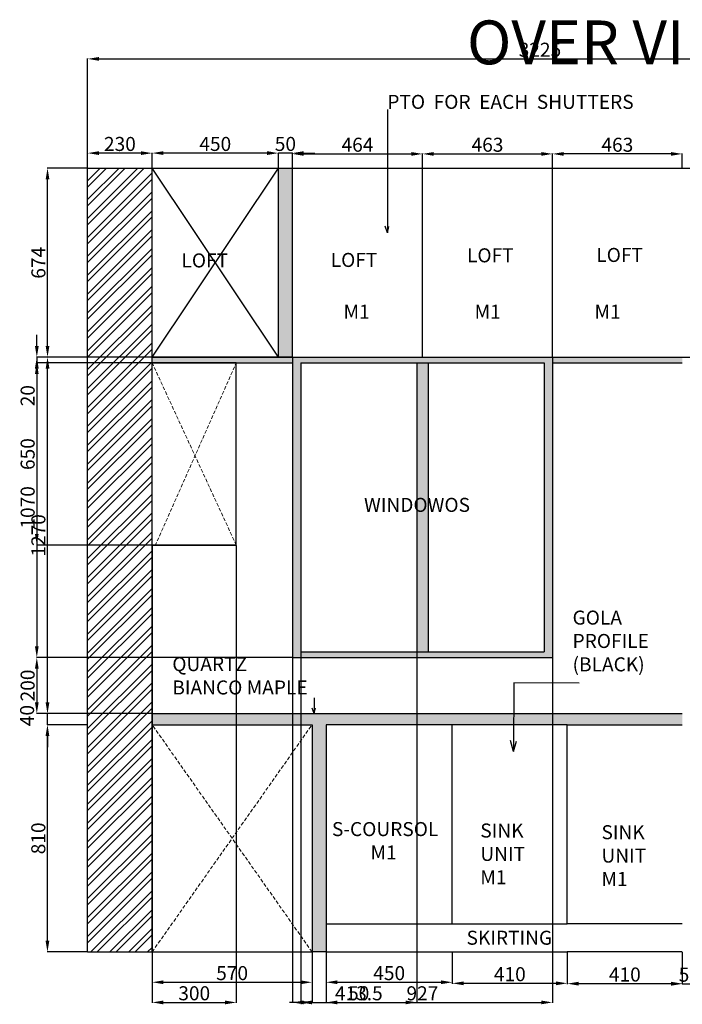
# Model space of a CAD drawing. Units: millimetres. Extents: x 144895 to 155057, y -2833 to 1092.
# Tile 1 of 4: x 144895 to 147257, y -2807 to 703. Entities that reach past the tile are written whole.
import ezdxf

# ---------------------------------------------------------------- set-up
doc = ezdxf.new("R2010")
doc.units = ezdxf.units.MM
doc.linetypes.add('DASHED', pattern=[19.05, 12.7, -6.35])
for name, color, linetype, lineweight in [('A-ANNO-DIMS', 2, 'Continuous', 18), ('A-ANNO-TEXT', 7, 'Continuous', 18), ('A-ELEV', 7, 'Continuous', 25), ('A-ELEV-HIDN', 8, 'DASHED', 18), ('A-ELEV-PATT', 252, 'Continuous', 13), ('A-WALL-PATT', 8, 'Continuous', 13)]:
    doc.layers.add(name, color=color, linetype=linetype, lineweight=lineweight)
doc.styles.get("Standard").update_dxf_attribs({"font": 'arial.ttf'})
doc.dimstyles.new('ISO-25', dxfattribs={"dimtxt": 50, "dimasz": 40, "dimexe": 1.25, "dimexo": 0.625, "dimtad": 1, "dimtxsty": 'Standard', "dimcen": 2.5, "dimadec": 0, "dimazin": 0, "dimtfac": 1, "dimtmove": 0, "dimatfit": 3, "dimfxl": 1, "dimarcsym": 0})

# ---------------------------------------------------------------- blocks, each defined once
blk = doc.blocks.new('*D10')
at = {"layer": 'A-ANNO-DIMS', "color": 0, "lineweight": -2, "transparency": 16777216}
for p, q in [((145367.5, -2621.3), (145367.5, -2730)), ((145937.5, -2621.3), (145937.5, -2730)), ((145407.5, -2728.8), (145897.5, -2728.8))]:
    blk.add_line(p, q, dxfattribs=at)
at = {"layer": 'A-ANNO-DIMS', "color": 0, "transparency": 16777216}
for points in [[(145407.5, -2722.1), (145407.5, -2735.4), (145367.5, -2728.8)], [(145897.5, -2722.1), (145897.5, -2735.4), (145937.5, -2728.8)]]:
    blk.add_solid(points, dxfattribs=at)
at = {"layer": 'Defpoints', "color": 0, "transparency": 16777216}
for p in [(145367.5, -2620.7), (145937.5, -2620.7), (145937.5, -2728.8)]:
    blk.add_point(p, dxfattribs=at)
at = {"layer": 'A-ANNO-DIMS', "color": 0, "transparency": 16777216, "insert": (145652.5, -2702.6), "char_height": 50, "attachment_point": 5}
blk.add_mtext('570', dxfattribs=at)
blk = doc.blocks.new('*D11')
at = {"layer": 'A-ANNO-DIMS', "color": 0, "lineweight": -2, "transparency": 16777216}
for p, q in [((146437.5, -2621.3), (146437.5, -2733.8)), ((146847.5, -2621.3), (146847.5, -2733.8)), ((146477.5, -2732.5), (146807.5, -2732.5))]:
    blk.add_line(p, q, dxfattribs=at)
at = {"layer": 'A-ANNO-DIMS', "color": 0, "transparency": 16777216}
for points in [[(146477.5, -2725.9), (146477.5, -2739.2), (146437.5, -2732.5)], [(146807.5, -2725.9), (146807.5, -2739.2), (146847.5, -2732.5)]]:
    blk.add_solid(points, dxfattribs=at)
at = {"layer": 'Defpoints', "color": 0, "transparency": 16777216}
for p in [(146437.5, -2620.7), (146847.5, -2620.7), (146847.5, -2732.5)]:
    blk.add_point(p, dxfattribs=at)
at = {"layer": 'A-ANNO-DIMS', "color": 0, "transparency": 16777216, "insert": (146642.5, -2706.4), "char_height": 50, "attachment_point": 5}
blk.add_mtext('410', dxfattribs=at)
blk = doc.blocks.new('*D12')
at = {"layer": 'A-ANNO-DIMS', "color": 0, "lineweight": -2, "transparency": 16777216}
for p, q in [((145987.5, -2621.3), (145987.5, -2730)), ((146437.5, -2621.3), (146437.5, -2730)), ((146027.5, -2728.8), (146397.5, -2728.8))]:
    blk.add_line(p, q, dxfattribs=at)
at = {"layer": 'A-ANNO-DIMS', "color": 0, "transparency": 16777216}
for points in [[(146027.5, -2722.1), (146027.5, -2735.4), (145987.5, -2728.8)], [(146397.5, -2722.1), (146397.5, -2735.4), (146437.5, -2728.8)]]:
    blk.add_solid(points, dxfattribs=at)
at = {"layer": 'Defpoints', "color": 0, "transparency": 16777216}
for p in [(145987.5, -2620.7), (146437.5, -2620.7), (146437.5, -2728.8)]:
    blk.add_point(p, dxfattribs=at)
at = {"layer": 'A-ANNO-DIMS', "color": 0, "transparency": 16777216, "insert": (146212.5, -2702.6), "char_height": 50, "attachment_point": 5}
blk.add_mtext('450', dxfattribs=at)
blk = doc.blocks.new('*D13')
at = {"layer": 'A-ANNO-DIMS', "color": 0, "lineweight": -2, "transparency": 16777216}
for p, q in [((147257.5, -2621.3), (147257.5, -2735.6)), ((147307.5, -2621.3), (147307.5, -2735.6)), ((147217.5, -2734.4), (147177.5, -2734.4)), ((147257.5, -2734.4), (147307.5, -2734.4)), ((147347.5, -2734.4), (147387.5, -2734.4))]:
    blk.add_line(p, q, dxfattribs=at)
at = {"layer": 'A-ANNO-DIMS', "color": 0, "transparency": 16777216}
for points in [[(147217.5, -2727.7), (147217.5, -2741.1), (147257.5, -2734.4)], [(147347.5, -2727.7), (147347.5, -2741.1), (147307.5, -2734.4)]]:
    blk.add_solid(points, dxfattribs=at)
at = {"layer": 'Defpoints', "color": 0, "transparency": 16777216}
for p in [(147257.5, -2620.7), (147307.5, -2620.7), (147307.5, -2734.4)]:
    blk.add_point(p, dxfattribs=at)
at = {"layer": 'A-ANNO-DIMS', "color": 0, "transparency": 16777216, "insert": (147282.5, -2708.2), "char_height": 50, "attachment_point": 5}
blk.add_mtext('50', dxfattribs=at)
blk = doc.blocks.new('*D15')
at = {"layer": 'A-ANNO-DIMS', "color": 0, "lineweight": -2, "transparency": 16777216}
for p, q in [((146847.5, -2621.3), (146847.5, -2735)), ((147257.5, -2621.3), (147257.5, -2735)), ((147217.5, -2733.8), (146887.5, -2733.8))]:
    blk.add_line(p, q, dxfattribs=at)
at = {"layer": 'A-ANNO-DIMS', "color": 0, "transparency": 16777216}
for points in [[(146887.5, -2727.1), (146887.5, -2740.4), (146847.5, -2733.8)], [(147217.5, -2727.1), (147217.5, -2740.4), (147257.5, -2733.8)]]:
    blk.add_solid(points, dxfattribs=at)
at = {"layer": 'Defpoints', "color": 0, "transparency": 16777216}
for p in [(146847.5, -2620.7), (147257.5, -2620.7), (146847.5, -2733.8)]:
    blk.add_point(p, dxfattribs=at)
at = {"layer": 'A-ANNO-DIMS', "color": 0, "transparency": 16777216, "insert": (147052.5, -2707.6), "char_height": 50, "attachment_point": 5}
blk.add_mtext('410', dxfattribs=at)
blk = doc.blocks.new('*D16')
at = {"layer": 'A-ANNO-DIMS', "color": 0, "lineweight": -2, "transparency": 16777216}
for p, q in [((145136.8, -1810.7), (144993, -1810.7)), ((144994.2, -2580.7), (144994.2, -1850.7)), ((145136.8, -2620.7), (144993, -2620.7))]:
    blk.add_line(p, q, dxfattribs=at)
at = {"layer": 'A-ANNO-DIMS', "color": 0, "transparency": 16777216}
for points in [[(144987.6, -1850.7), (145000.9, -1850.7), (144994.2, -1810.7)], [(144987.6, -2580.7), (145000.9, -2580.7), (144994.2, -2620.7)]]:
    blk.add_solid(points, dxfattribs=at)
at = {"layer": 'Defpoints', "color": 0, "transparency": 16777216}
for p in [(144994.2, -1810.7), (145137.5, -1810.7), (145137.5, -2620.7)]:
    blk.add_point(p, dxfattribs=at)
at = {"layer": 'A-ANNO-DIMS', "color": 0, "transparency": 16777216, "insert": (144968.1, -2215.7), "char_height": 50, "attachment_point": 5, "rotation": 90}
blk.add_mtext('810', dxfattribs=at)
blk = doc.blocks.new('*D17')
at = {"layer": 'A-ANNO-DIMS', "color": 0, "lineweight": -2, "transparency": 16777216}
for p, q in [((144994.2, -1730.7), (144994.2, -1690.7)), ((145136.8, -1770.7), (144993, -1770.7)), ((144994.2, -1810.7), (144994.2, -1770.7)), ((145136.8, -1810.7), (144993, -1810.7)), ((144994.2, -1850.7), (144994.2, -1890.7))]:
    blk.add_line(p, q, dxfattribs=at)
at = {"layer": 'A-ANNO-DIMS', "color": 0, "transparency": 16777216}
for points in [[(144987.6, -1730.7), (145000.9, -1730.7), (144994.2, -1770.7)], [(144987.6, -1850.7), (145000.9, -1850.7), (144994.2, -1810.7)]]:
    blk.add_solid(points, dxfattribs=at)
at = {"layer": 'Defpoints', "color": 0, "transparency": 16777216}
for p in [(144994.2, -1770.7), (145137.5, -1770.7), (145137.5, -1810.7)]:
    blk.add_point(p, dxfattribs=at)
at = {"layer": 'A-ANNO-DIMS', "color": 0, "transparency": 16777216, "insert": (144928.1, -1778.1), "char_height": 50, "attachment_point": 5, "rotation": 90}
blk.add_mtext('40', dxfattribs=at)
blk = doc.blocks.new('*D18')
at = {"layer": 'A-ANNO-DIMS', "color": 0, "lineweight": -2, "ltscale": 20, "transparency": 16777216}
for p, q in [((145367.5, 173.9), (145367.5, 228.6)), ((145777.5, 227.3), (145407.5, 227.3)), ((145817.5, 173.9), (145817.5, 228.6))]:
    blk.add_line(p, q, dxfattribs=at)
at = {"layer": 'A-ANNO-DIMS', "color": 0, "ltscale": 20, "transparency": 16777216}
for points in [[(145407.5, 234), (145407.5, 220.7), (145367.5, 227.3)], [(145777.5, 234), (145777.5, 220.7), (145817.5, 227.3)]]:
    blk.add_solid(points, dxfattribs=at)
at = {"layer": 'Defpoints', "color": 0, "ltscale": 20, "transparency": 16777216}
for p in [(145367.5, 227.3), (145367.5, 173.3), (145817.5, 173.3)]:
    blk.add_point(p, dxfattribs=at)
at = {"layer": 'A-ANNO-DIMS', "color": 0, "ltscale": 20, "transparency": 16777216, "insert": (145592.5, 253.5), "char_height": 50, "attachment_point": 5}
blk.add_mtext('450', dxfattribs=at)
blk = doc.blocks.new('*D19')
at = {"layer": 'A-ANNO-DIMS', "color": 0, "lineweight": -2, "ltscale": 20, "transparency": 16777216}
for p, q in [((145777.5, 227.3), (145737.5, 227.3)), ((145817.5, 173.9), (145817.5, 228.6)), ((145867.5, 227.3), (145817.5, 227.3)), ((145867.5, 173.9), (145867.5, 228.6)), ((145907.5, 227.3), (145947.5, 227.3))]:
    blk.add_line(p, q, dxfattribs=at)
at = {"layer": 'A-ANNO-DIMS', "color": 0, "ltscale": 20, "transparency": 16777216}
for points in [[(145777.5, 234), (145777.5, 220.7), (145817.5, 227.3)], [(145907.5, 234), (145907.5, 220.7), (145867.5, 227.3)]]:
    blk.add_solid(points, dxfattribs=at)
at = {"layer": 'Defpoints', "color": 0, "ltscale": 20, "transparency": 16777216}
for p in [(145817.5, 227.3), (145817.5, 173.3), (145867.5, 173.3)]:
    blk.add_point(p, dxfattribs=at)
at = {"layer": 'A-ANNO-DIMS', "color": 0, "ltscale": 20, "transparency": 16777216, "insert": (145842.5, 253.5), "char_height": 50, "attachment_point": 5}
blk.add_mtext('50', dxfattribs=at)
blk = doc.blocks.new('*D20')
at = {"layer": 'A-ANNO-DIMS', "color": 0, "lineweight": -2, "ltscale": 20, "transparency": 16777216}
for p, q in [((145867.5, 173.9), (145867.5, 225.7)), ((145907.5, 224.4), (146291.5, 224.4)), ((146331.5, 173.9), (146331.5, 225.7))]:
    blk.add_line(p, q, dxfattribs=at)
at = {"layer": 'A-ANNO-DIMS', "color": 0, "ltscale": 20, "transparency": 16777216}
for points in [[(145907.5, 231.1), (145907.5, 217.7), (145867.5, 224.4)], [(146291.5, 231.1), (146291.5, 217.7), (146331.5, 224.4)]]:
    blk.add_solid(points, dxfattribs=at)
at = {"layer": 'Defpoints', "color": 0, "ltscale": 20, "transparency": 16777216}
for p in [(146331.5, 224.4), (145867.5, 173.3), (146331.5, 173.3)]:
    blk.add_point(p, dxfattribs=at)
at = {"layer": 'A-ANNO-DIMS', "color": 0, "ltscale": 20, "transparency": 16777216, "insert": (146099.5, 250.6), "char_height": 50, "attachment_point": 5}
blk.add_mtext('464', dxfattribs=at)
blk = doc.blocks.new('*D21')
at = {"layer": 'A-ANNO-DIMS', "color": 0, "lineweight": -2, "ltscale": 20, "transparency": 16777216}
for p, q in [((146331.5, 173.9), (146331.5, 225.6)), ((146371.5, 224.4), (146754.5, 224.4)), ((146794.5, 173.9), (146794.5, 225.6))]:
    blk.add_line(p, q, dxfattribs=at)
at = {"layer": 'A-ANNO-DIMS', "color": 0, "ltscale": 20, "transparency": 16777216}
for points in [[(146371.5, 231), (146371.5, 217.7), (146331.5, 224.4)], [(146754.5, 231), (146754.5, 217.7), (146794.5, 224.4)]]:
    blk.add_solid(points, dxfattribs=at)
at = {"layer": 'Defpoints', "color": 0, "ltscale": 20, "transparency": 16777216}
for p in [(146794.5, 224.4), (146331.5, 173.3), (146794.5, 173.3)]:
    blk.add_point(p, dxfattribs=at)
at = {"layer": 'A-ANNO-DIMS', "color": 0, "ltscale": 20, "transparency": 16777216, "insert": (146563, 250.6), "char_height": 50, "attachment_point": 5}
blk.add_mtext('463', dxfattribs=at)
blk = doc.blocks.new('*D22')
at = {"layer": 'A-ANNO-DIMS', "color": 0, "lineweight": -2, "ltscale": 20, "transparency": 16777216}
for p, q in [((146794.5, 173.9), (146794.5, 225.6)), ((147217.5, 224.4), (146834.5, 224.4)), ((147257.5, 173.9), (147257.5, 225.6))]:
    blk.add_line(p, q, dxfattribs=at)
at = {"layer": 'A-ANNO-DIMS', "color": 0, "ltscale": 20, "transparency": 16777216}
for points in [[(146834.5, 231), (146834.5, 217.7), (146794.5, 224.4)], [(147217.5, 231), (147217.5, 217.7), (147257.5, 224.4)]]:
    blk.add_solid(points, dxfattribs=at)
at = {"layer": 'Defpoints', "color": 0, "ltscale": 20, "transparency": 16777216}
for p in [(146794.5, 224.4), (146794.5, 173.3), (147257.5, 173.3)]:
    blk.add_point(p, dxfattribs=at)
at = {"layer": 'A-ANNO-DIMS', "color": 0, "ltscale": 20, "transparency": 16777216, "insert": (147026, 250.6), "char_height": 50, "attachment_point": 5}
blk.add_mtext('463', dxfattribs=at)
blk = doc.blocks.new('*D23')
at = {"layer": 'A-ANNO-DIMS', "color": 0, "lineweight": -2, "ltscale": 20, "transparency": 16777216}
for p, q in [((145137.5, 173.9), (145137.5, 228.5)), ((145327.5, 227.2), (145177.5, 227.2)), ((145367.5, 173.9), (145367.5, 228.5))]:
    blk.add_line(p, q, dxfattribs=at)
at = {"layer": 'A-ANNO-DIMS', "color": 0, "ltscale": 20, "transparency": 16777216}
for points in [[(145177.5, 233.9), (145177.5, 220.5), (145137.5, 227.2)], [(145327.5, 233.9), (145327.5, 220.5), (145367.5, 227.2)]]:
    blk.add_solid(points, dxfattribs=at)
at = {"layer": 'Defpoints', "color": 0, "ltscale": 20, "transparency": 16777216}
for p in [(145137.5, 227.2), (145137.5, 173.3), (145367.5, 173.3)]:
    blk.add_point(p, dxfattribs=at)
at = {"layer": 'A-ANNO-DIMS', "color": 0, "ltscale": 20, "transparency": 16777216, "insert": (145252.5, 253.4), "char_height": 50, "attachment_point": 5}
blk.add_mtext('230', dxfattribs=at)
blk = doc.blocks.new('*D28')
at = {"layer": 'A-ANNO-DIMS', "color": 0, "lineweight": -2, "ltscale": 20, "transparency": 16777216}
for p, q in [((145136.8, -500.7), (144993.3, -500.7)), ((144994.5, -1730.7), (144994.5, -540.7)), ((145129.6, -1770.7), (144993.3, -1770.7))]:
    blk.add_line(p, q, dxfattribs=at)
at = {"layer": 'A-ANNO-DIMS', "color": 0, "ltscale": 20, "transparency": 16777216}
for points in [[(144987.9, -540.7), (145001.2, -540.7), (144994.5, -500.7)], [(144987.9, -1730.7), (145001.2, -1730.7), (144994.5, -1770.7)]]:
    blk.add_solid(points, dxfattribs=at)
at = {"layer": 'Defpoints', "color": 0, "ltscale": 20, "transparency": 16777216}
for p in [(144994.5, -500.7), (145137.5, -500.7), (145130.3, -1770.7)]:
    blk.add_point(p, dxfattribs=at)
at = {"layer": 'A-ANNO-DIMS', "color": 0, "ltscale": 20, "transparency": 16777216, "insert": (144968.4, -1135.7), "char_height": 50, "attachment_point": 5, "rotation": 90}
blk.add_mtext('1270', dxfattribs=at)
blk = doc.blocks.new('*D29')
at = {"layer": 'A-ANNO-DIMS', "color": 0, "lineweight": -2, "ltscale": 20, "transparency": 16777216}
for p, q in [((145136.8, 173.3), (144993.3, 173.3)), ((144994.5, -460.7), (144994.5, 133.3)), ((145136.8, -500.7), (144993.3, -500.7))]:
    blk.add_line(p, q, dxfattribs=at)
at = {"layer": 'A-ANNO-DIMS', "color": 0, "ltscale": 20, "transparency": 16777216}
for points in [[(144987.9, 133.3), (145001.2, 133.3), (144994.5, 173.3)], [(144987.9, -460.7), (145001.2, -460.7), (144994.5, -500.7)]]:
    blk.add_solid(points, dxfattribs=at)
at = {"layer": 'Defpoints', "color": 0, "ltscale": 20, "transparency": 16777216}
for p in [(144994.5, 173.3), (145137.5, 173.3), (145137.5, -500.7)]:
    blk.add_point(p, dxfattribs=at)
at = {"layer": 'A-ANNO-DIMS', "color": 0, "ltscale": 20, "transparency": 16777216, "insert": (144968.4, -163.7), "char_height": 50, "attachment_point": 5, "rotation": 90}
blk.add_mtext('674', dxfattribs=at)
blk = doc.blocks.new('*D46')
at = {"layer": 'A-ANNO-DIMS', "color": 0, "lineweight": -2, "ltscale": 20, "transparency": 16777216}
for p, q in [((145137.5, 173.9), (145137.5, 564.4)), ((145177.5, 563.2), (148322.5, 563.2)), ((148362.5, 173.9), (148362.5, 564.4))]:
    blk.add_line(p, q, dxfattribs=at)
at = {"layer": 'A-ANNO-DIMS', "color": 0, "ltscale": 20, "transparency": 16777216}
for points in [[(145177.5, 569.8), (145177.5, 556.5), (145137.5, 563.2)], [(148322.5, 569.8), (148322.5, 556.5), (148362.5, 563.2)]]:
    blk.add_solid(points, dxfattribs=at)
at = {"layer": 'Defpoints', "color": 0, "ltscale": 20, "transparency": 16777216}
for p in [(148362.5, 563.2), (145137.5, 173.3), (148362.5, 173.3)]:
    blk.add_point(p, dxfattribs=at)
at = {"layer": 'A-ANNO-DIMS', "color": 0, "ltscale": 20, "transparency": 16777216, "insert": (146750, 589.4), "char_height": 50, "attachment_point": 5}
blk.add_mtext('3225', dxfattribs=at)
blk = doc.blocks.new('*D48')
at = {"layer": 'A-ANNO-DIMS', "color": 0, "lineweight": -2, "ltscale": 20, "transparency": 16777216}
for p, q in [((145867.5, -1571.3), (145867.5, -2802)), ((146794.5, -1571.3), (146794.5, -2802)), ((145907.5, -2800.7), (146754.5, -2800.7))]:
    blk.add_line(p, q, dxfattribs=at)
at = {"layer": 'A-ANNO-DIMS', "color": 0, "ltscale": 20, "transparency": 16777216}
for points in [[(145907.5, -2794), (145907.5, -2807.4), (145867.5, -2800.7)], [(146754.5, -2794), (146754.5, -2807.4), (146794.5, -2800.7)]]:
    blk.add_solid(points, dxfattribs=at)
at = {"layer": 'Defpoints', "color": 0, "ltscale": 20, "transparency": 16777216}
for p in [(145867.5, -1570.7), (146794.5, -1570.7), (146794.5, -2800.7)]:
    blk.add_point(p, dxfattribs=at)
at = {"layer": 'A-ANNO-DIMS', "color": 0, "ltscale": 20, "transparency": 16777216, "insert": (146331, -2774.6), "char_height": 50, "attachment_point": 5}
blk.add_mtext('927', dxfattribs=at)
blk = doc.blocks.new('*D49')
at = {"layer": 'A-ANNO-DIMS', "color": 0, "lineweight": -2, "ltscale": 20, "transparency": 16777216}
for p, q in [((145897.5, -1551.3), (145897.5, -2802)), ((146311, -1551.3), (146311, -2802)), ((145937.5, -2800.7), (146271, -2800.7))]:
    blk.add_line(p, q, dxfattribs=at)
at = {"layer": 'A-ANNO-DIMS', "color": 0, "ltscale": 20, "transparency": 16777216}
for points in [[(145937.5, -2794), (145937.5, -2807.4), (145897.5, -2800.7)], [(146271, -2794), (146271, -2807.4), (146311, -2800.7)]]:
    blk.add_solid(points, dxfattribs=at)
at = {"layer": 'Defpoints', "color": 0, "ltscale": 20, "transparency": 16777216}
for p in [(145897.5, -1550.7), (146311, -1550.7), (146311, -2800.7)]:
    blk.add_point(p, dxfattribs=at)
at = {"layer": 'A-ANNO-DIMS', "color": 0, "ltscale": 20, "transparency": 16777216, "insert": (146104.2, -2774.5), "char_height": 50, "attachment_point": 5}
blk.add_mtext('413.5', dxfattribs=at)
blk = doc.blocks.new('*D50')
at = {"layer": 'A-ANNO-DIMS', "color": 0, "lineweight": -2, "ltscale": 20, "transparency": 16777216}
for p, q in [((145866.8, -500.7), (144955, -500.7)), ((144956.3, -540.7), (144956.3, -1530.7)), ((145866.8, -1570.7), (144955, -1570.7))]:
    blk.add_line(p, q, dxfattribs=at)
at = {"layer": 'A-ANNO-DIMS', "color": 0, "ltscale": 20, "transparency": 16777216}
for points in [[(144949.6, -540.7), (144963, -540.7), (144956.3, -500.7)], [(144949.6, -1530.7), (144963, -1530.7), (144956.3, -1570.7)]]:
    blk.add_solid(points, dxfattribs=at)
at = {"layer": 'Defpoints', "color": 0, "ltscale": 20, "transparency": 16777216}
for p in [(145867.5, -500.7), (144956.3, -1570.7), (145867.5, -1570.7)]:
    blk.add_point(p, dxfattribs=at)
at = {"layer": 'A-ANNO-DIMS', "color": 0, "ltscale": 20, "transparency": 16777216, "insert": (144930.1, -1035.7), "char_height": 50, "attachment_point": 5, "rotation": 90}
blk.add_mtext('1070', dxfattribs=at)
blk = doc.blocks.new('*D51')
at = {"layer": 'A-ANNO-DIMS', "color": 0, "lineweight": -2, "ltscale": 20, "transparency": 16777216}
for p, q in [((145866.8, -1570.7), (144955, -1570.7)), ((144956.3, -1610.7), (144956.3, -1730.7)), ((145366.8, -1770.7), (144955, -1770.7))]:
    blk.add_line(p, q, dxfattribs=at)
at = {"layer": 'A-ANNO-DIMS', "color": 0, "ltscale": 20, "transparency": 16777216}
for points in [[(144949.6, -1610.7), (144963, -1610.7), (144956.3, -1570.7)], [(144949.6, -1730.7), (144963, -1730.7), (144956.3, -1770.7)]]:
    blk.add_solid(points, dxfattribs=at)
at = {"layer": 'Defpoints', "color": 0, "ltscale": 20, "transparency": 16777216}
for p in [(145867.5, -1570.7), (144956.3, -1770.7), (145367.5, -1770.7)]:
    blk.add_point(p, dxfattribs=at)
at = {"layer": 'A-ANNO-DIMS', "color": 0, "ltscale": 20, "transparency": 16777216, "insert": (144930.1, -1670.7), "char_height": 50, "attachment_point": 5, "rotation": 90}
blk.add_mtext('200', dxfattribs=at)
blk = doc.blocks.new('*D52')
at = {"layer": 'A-ANNO-DIMS', "color": 0, "lineweight": -2, "ltscale": 20, "transparency": 16777216}
for p, q in [((145367.5, -1171.3), (145367.5, -2802)), ((145667.5, -1171.3), (145667.5, -2802)), ((145407.5, -2800.7), (145627.5, -2800.7))]:
    blk.add_line(p, q, dxfattribs=at)
at = {"layer": 'A-ANNO-DIMS', "color": 0, "ltscale": 20, "transparency": 16777216}
for points in [[(145407.5, -2794), (145407.5, -2807.4), (145367.5, -2800.7)], [(145627.5, -2794), (145627.5, -2807.4), (145667.5, -2800.7)]]:
    blk.add_solid(points, dxfattribs=at)
at = {"layer": 'Defpoints', "color": 0, "ltscale": 20, "transparency": 16777216}
for p in [(145367.5, -1170.7), (145667.5, -1170.7), (145667.5, -2800.7)]:
    blk.add_point(p, dxfattribs=at)
at = {"layer": 'A-ANNO-DIMS', "color": 0, "ltscale": 20, "transparency": 16777216, "insert": (145517.5, -2774.5), "char_height": 50, "attachment_point": 5}
blk.add_mtext('300', dxfattribs=at)
blk = doc.blocks.new('*D53')
at = {"layer": 'A-ANNO-DIMS', "color": 0, "lineweight": -2, "ltscale": 20, "transparency": 16777216}
for p, q in [((145666.8, -520.7), (144955, -520.7)), ((144956.3, -560.7), (144956.3, -1130.7)), ((145666.8, -1170.7), (144955, -1170.7))]:
    blk.add_line(p, q, dxfattribs=at)
at = {"layer": 'A-ANNO-DIMS', "color": 0, "ltscale": 20, "transparency": 16777216}
for points in [[(144949.6, -560.7), (144963, -560.7), (144956.3, -520.7)], [(144949.6, -1130.7), (144963, -1130.7), (144956.3, -1170.7)]]:
    blk.add_solid(points, dxfattribs=at)
at = {"layer": 'Defpoints', "color": 0, "ltscale": 20, "transparency": 16777216}
for p in [(145667.5, -520.7), (144956.3, -1170.7), (145667.5, -1170.7)]:
    blk.add_point(p, dxfattribs=at)
at = {"layer": 'A-ANNO-DIMS', "color": 0, "ltscale": 20, "transparency": 16777216, "insert": (144930.1, -845.7), "char_height": 50, "attachment_point": 5, "rotation": 90}
blk.add_mtext('650', dxfattribs=at)
blk = doc.blocks.new('*D55')
at = {"layer": 'A-ANNO-DIMS', "color": 0, "lineweight": -2, "ltscale": 20, "transparency": 16777216}
for p, q in [((144956.3, -460.7), (144956.3, -420.7)), ((145366.8, -500.7), (144955, -500.7)), ((145366.8, -520.7), (144955, -520.7)), ((144956.3, -500.7), (144956.3, -520.7)), ((144956.3, -560.7), (144956.3, -674.3))]:
    blk.add_line(p, q, dxfattribs=at)
at = {"layer": 'A-ANNO-DIMS', "color": 0, "ltscale": 20, "transparency": 16777216}
for points in [[(144949.6, -460.7), (144963, -460.7), (144956.3, -500.7)], [(144949.6, -560.7), (144963, -560.7), (144956.3, -520.7)]]:
    blk.add_solid(points, dxfattribs=at)
at = {"layer": 'Defpoints', "color": 0, "ltscale": 20, "transparency": 16777216}
for p in [(144956.3, -520.7), (145367.5, -500.7), (145367.5, -520.7)]:
    blk.add_point(p, dxfattribs=at)
at = {"layer": 'A-ANNO-DIMS', "color": 0, "ltscale": 20, "transparency": 16777216, "insert": (144930.1, -637.5), "char_height": 50, "attachment_point": 5, "rotation": 90}
blk.add_mtext('20', dxfattribs=at)
blk = doc.blocks.new('*D57')
at = {"layer": 'A-ANNO-DIMS', "color": 0, "lineweight": -2, "ltscale": 20, "transparency": 16777216}
for p, q in [((145937.5, -1811.3), (145937.5, -2802)), ((145987.5, -1811.3), (145987.5, -2802)), ((145897.5, -2800.7), (145857.5, -2800.7)), ((145937.5, -2800.7), (145987.5, -2800.7)), ((146027.5, -2800.7), (146140.2, -2800.7))]:
    blk.add_line(p, q, dxfattribs=at)
at = {"layer": 'A-ANNO-DIMS', "color": 0, "ltscale": 20, "transparency": 16777216}
for points in [[(145897.5, -2794), (145897.5, -2807.4), (145937.5, -2800.7)], [(146027.5, -2794), (146027.5, -2807.4), (145987.5, -2800.7)]]:
    blk.add_solid(points, dxfattribs=at)
at = {"layer": 'Defpoints', "color": 0, "ltscale": 20, "transparency": 16777216}
for p in [(145937.5, -1810.7), (145987.5, -1810.7), (145987.5, -2800.7)]:
    blk.add_point(p, dxfattribs=at)
at = {"layer": 'A-ANNO-DIMS', "color": 0, "ltscale": 20, "transparency": 16777216, "insert": (146103.8, -2774.6), "char_height": 50, "attachment_point": 5}
blk.add_mtext('50', dxfattribs=at)

msp = doc.modelspace()

# ---------------------------------------------------------------- hatches: boundary and pattern name
at = {"layer": 'A-ELEV-PATT', "ltscale": 20}
h = msp.add_hatch(color=256, dxfattribs=at)
h.dxf.hatch_style = 1
h.paths.add_polyline_path([(146350.96, -520.704), (146310.96, -520.704), (146310.96, -1550.704), (146350.96, -1550.704)])
h.paths.add_polyline_path([(145867.46, 173.296), (145817.46, 173.296), (145817.46, -500.704), (145867.46, -500.704)])
h.paths.add_polyline_path([(145867.46, -500.704), (145367.46, -500.704), (145367.46, -520.704), (145867.46, -520.704)])
h.paths.add_polyline_path([(147257.46, -500.704), (146794.46, -500.704), (146794.46, -520.704), (147257.46, -520.704)])
h.paths.add_polyline_path([(147257.46, -1770.704), (146656.275, -1770.704), (146656.07, -1810.704), (146847.46, -1810.704), (147257.46, -1810.704)])
h.paths.add_polyline_path([(148132.46, -550.704), (148082.46, -550.704), (148082.46, -2610.704), (147307.46, -2610.704), (147307.46, -2620.704), (148132.46, -2620.704)])
h.paths.add_polyline_path([(146109.393, -1080.003), (146541.794, -1080.003), (146541.794, -976.968), (146109.393, -976.968)], flags=9)
h = msp.add_hatch(color=256, dxfattribs=at)
h.dxf.hatch_style = 1
h.paths.add_polyline_path([(146794.46, -500.704), (145867.46, -500.704), (145867.46, -1570.704), (146794.46, -1570.704)])
h.paths.add_polyline_path([(145897.46, -520.704), (146764.46, -520.704), (146764.46, -1550.704), (145897.46, -1550.704)], flags=16)
h.paths.add_polyline_path([(146350.96, -520.704), (146310.96, -520.704), (146310.96, -1550.704), (146350.96, -1550.704)], flags=0)
h.paths.add_polyline_path([(146109.393, -1080.003), (146541.794, -1080.003), (146541.794, -976.968), (146109.393, -976.968)], flags=8)
h = msp.add_hatch(color=256, dxfattribs=at)
h.dxf.hatch_style = 1
h.paths.add_polyline_path([(145987.46, -1810.704), (146437.46, -1810.704), (146656.07, -1810.704), (146656.275, -1770.704), (145367.46, -1770.704), (145367.46, -1810.704), (145937.46, -1810.704), (145937.46, -2620.704), (145987.46, -2620.704)])
at = {"layer": 'A-WALL-PATT'}
h = msp.add_hatch(dxfattribs=at)
h.set_pattern_fill('ANSI32', color=256, scale=5)
h.paths.add_polyline_path([(145137.46, -1770.704), (145137.46, -2620.704), (145367.46, -2620.704), (145367.46, -1770.704), (145367.46, 173.296), (145137.46, 173.296), (145137.46, -500.704)])

# ---------------------------------------------------------------- linework, layer by layer
at = {"layer": 'A-ELEV', "ltscale": 20}
for p, q in [((146205.92, 383.182), (146205.92, -56.801)), ((145817.46, -500.704), (145367.46, 173.296)), ((145367.46, -500.704), (145817.46, 173.296)), ((146205.92, -56.801), (146198.728, -33.397)), ((146205.92, -56.801), (146211.147, -34.012)), ((145867.46, -500.704), (145867.46, -1570.704)), ((145897.46, -520.704), (145897.46, -1550.704)), ((146310.96, -520.704), (146310.96, -1550.704)), ((146350.96, -520.704), (146350.96, -1550.704)), ((146764.46, -520.704), (146764.46, -1550.704)), ((146794.46, -500.704), (146794.46, -1570.704)), ((146656.835, -1661.386), (146655.58, -1906.229)), ((146889.947, -1662.581), (146656.835, -1661.386)), ((145944.757, -1715.038), (145944.757, -1770.704)), ((145944.757, -1770.704), (145938.059, -1751.315)), ((145944.757, -1770.704), (145949.791, -1751.784)), ((146655.58, -1906.229), (146644.8, -1867.446)), ((146655.58, -1906.229), (146666.226, -1868.708)), ((145987.46, -2620.704), (145937.46, -2620.704))]:
    msp.add_line(p, q, dxfattribs=at)
at = {"layer": 'A-ELEV'}
for p, q in [((145137.46, 173.296), (148362.46, 173.296)), ((145137.46, -500.704), (145137.46, 173.296)), ((145367.46, -1770.704), (145367.46, 173.296)), ((145817.46, -500.704), (145817.46, 173.296)), ((145867.46, -500.704), (145867.46, 173.296)), ((146331.46, -500.704), (146331.46, 173.296)), ((146794.46, -500.704), (146794.46, 173.296)), ((145136.298, -520.704), (145137.46, -520.704)), ((145137.46, -1770.704), (145137.46, -500.704)), ((145367.46, -500.704), (148131.298, -500.704)), ((145367.46, -520.704), (145867.46, -520.704)), ((145667.46, -1170.704), (145667.46, -520.704)), ((145897.46, -520.704), (146764.46, -520.704)), ((146794.46, -520.704), (147257.46, -520.704)), ((145367.46, -1170.704), (145667.46, -1170.704)), ((145867.46, -1570.704), (146794.46, -1570.704)), ((145897.46, -1550.704), (146764.46, -1550.704)), ((145137.46, -2620.704), (145137.46, -1770.704)), ((145367.46, -2620.704), (145367.46, -1770.704)), ((145367.46, -1770.704), (147257.46, -1770.704)), ((145367.46, -1810.704), (145937.46, -1810.704)), ((145937.46, -1810.704), (145937.46, -2620.704)), ((145987.46, -1810.704), (145987.46, -2620.704)), ((146437.46, -1810.704), (145987.46, -1810.704)), ((146437.46, -2520.704), (146437.46, -1810.704)), ((146847.46, -1810.704), (146437.46, -1810.704)), ((146847.46, -2520.704), (146847.46, -1810.704)), ((146847.46, -1810.704), (147257.46, -1810.704)), ((145987.46, -2520.704), (146437.46, -2520.704)), ((146437.46, -2520.704), (146847.46, -2520.704)), ((147257.46, -2520.704), (146847.46, -2520.704)), ((145137.46, -2620.704), (145937.46, -2620.704)), ((145987.46, -2620.704), (146437.46, -2620.704)), ((146437.46, -2620.704), (146847.46, -2620.704)), ((147257.46, -2620.704), (146847.46, -2620.704))]:
    msp.add_line(p, q, dxfattribs=at)
at = {"layer": 'A-ELEV-HIDN'}
for p, q in [((145667.46, -1170.704), (145367.46, -520.704)), ((145378.207, -1172.824), (145667.46, -520.704)), ((145937.46, -2620.704), (145367.46, -1810.704)), ((145367.46, -2620.704), (145937.46, -1810.704))]:
    msp.add_line(p, q, dxfattribs=at)

# ---------------------------------------------------------------- texts
at = {"layer": 'A-ANNO-TEXT', "attachment_point": 1}
for s, width, gutter_width, insert, char_height in [('OVER VIEW', 9064.84564, 39.102, (146489.911, 700.132), 156.408), ('PTO  FOR  EACH  SHUTTERS', 2897.81963, 12.5, (146205.92, 434.922), 50), ('LOFT ', 2897.81963, 12.5, (145472.006, -130.379), 50), ('LOFT ', 2897.81963, 12.5, (146004.094, -128.541), 50), ('LOFT ', 2897.81963, 12.5, (146489.911, -112.177), 50), ('LOFT ', 2897.81963, 12.5, (146950.908, -110.81), 50), ('M1 ', 2897.81963, 12.5, (146049.788, -313.072), 50), ('M1 ', 2897.81963, 12.5, (146516.89, -313.072), 50), ('M1 ', 2897.81963, 12.5, (146944.502, -313.072), 50), ('WINDOWOS', 2897.81963, 12.5, (146122.746, -1001.814), 50), ('GOLA \\PPROFILE \\P(BLACK)', 2897.81963, 12.5, (146866.225, -1403.708), 50), ('QUARTZ\\PBIANCO MAPLE', 2897.81963, 12.5, (145439.407, -1569.47), 50), ('\\PS-COURSOL\\P         M1', 2897.81963, 12.5, (146008.452, -2074.351), 50), ('\\PSINK \\PUNIT  \\PM1', 2897.81963, 12.5, (146537.356, -2079.433), 50), ('\\PSINK \\PUNIT  \\PM1', 2897.81963, 12.5, (146969.285, -2085.423), 50), ('SKIRTING', 2897.81963, 12.5, (146488.274, -2545.02), 50)]:
    msp.add_mtext_dynamic_manual_height_columns(s, width=width, gutter_width=gutter_width, heights=[0], dxfattribs=dict(at, insert=insert, char_height=char_height))

# ---------------------------------------------------------------- dimensions: what is measured, and where the dimension line sits
at = {"layer": 'A-ANNO-DIMS', "ltscale": 20}
for base, p1, p2, override, picture, middle in [((148362.46, 563.182), (145137.46, 173.296), (148362.46, 173.296), {"dimdec": 0, "dimlfac": 1, "dimrnd": 0, "dimzin": 0, "dimdsep": 46, "dimlunit": 2}, '*D46', (146749.96, 589.353)), ((145137.46, 227.21), (145367.46, 173.296), (145137.46, 173.296), {"dimclrd": 0, "dimclre": 0, "dimclrt": 0}, '*D23', (145252.46, 253.381)), ((145367.46, 227.346), (145817.46, 173.296), (145367.46, 173.296), {"dimclrd": 0, "dimclre": 0, "dimclrt": 0}, '*D18', (145592.46, 253.5)), ((146331.46, 224.415), (145867.46, 173.296), (146331.46, 173.296), {"dimclrd": 0, "dimclre": 0, "dimclrt": 0}, '*D20', (146099.46, 250.568)), ((146794.46, 224.38), (146331.46, 173.296), (146794.46, 173.296), {"dimclrd": 0, "dimclre": 0, "dimclrt": 0}, '*D21', (146562.96, 250.551)), ((146794.46, 224.38), (147257.46, 173.296), (146794.46, 173.296), {"dimclrd": 0, "dimclre": 0, "dimclrt": 0}, '*D22', (147025.96, 250.551)), ((145667.46, -2800.704), (145367.46, -1170.704), (145667.46, -1170.704), {"dimdec": 0, "dimlfac": 1, "dimrnd": 0, "dimzin": 0, "dimdsep": 46, "dimlunit": 2}, '*D52', (145517.46, -2774.533)), ((146794.46, -2800.704), (145867.46, -1570.704), (146794.46, -1570.704), {"dimdec": 0, "dimlfac": 1, "dimrnd": 0, "dimzin": 0, "dimdsep": 46, "dimlunit": 2}, '*D48', (146330.96, -2774.55)), ((146310.96, -2800.704), (145897.46, -1550.704), (146310.96, -1550.704), {"dimdec": 1, "dimlfac": 1, "dimrnd": 0, "dimzin": 0, "dimdsep": 46, "dimlunit": 2}, '*D49', (146104.21, -2774.533)), ((145987.46, -2800.704), (145937.46, -1810.704), (145987.46, -1810.704), {"dimdec": 0, "dimlfac": 1, "dimrnd": 0, "dimzin": 0, "dimdsep": 46, "dimlunit": 2}, '*D57', (146103.812, -2774.55))]:
    dim = msp.add_linear_dim(base=base, p1=p1, p2=p2, dimstyle='ISO-25', override=override, dxfattribs=at)
    dim.commit()
    dim.dimension.update_dxf_attribs({"geometry": picture, "text_midpoint": middle})
dim = msp.add_linear_dim(base=(145817.46, 227.346), p1=(145867.46, 173.296), p2=(145817.46, 173.296), dimstyle='ISO-25', override={"dimclrd": 0, "dimclre": 0, "dimclrt": 0}, dxfattribs=at)
dim.commit()
dim.dimension.update_dxf_attribs({"geometry": '*D19', "text_midpoint": (145842.46, 227.346), "dimtype": 160})
for base, p1, p2, override, picture, middle in [((144994.528, 173.296), (145137.46, -500.704), (145137.46, 173.296), {"dimclrd": 0, "dimclre": 0, "dimclrt": 0}, '*D29', (144968.375, -163.704)), ((144956.298, -520.704), (145367.46, -500.704), (145367.46, -520.704), {"dimdec": 0, "dimlfac": 1, "dimrnd": 0, "dimzin": 0, "dimdsep": 46, "dimlunit": 2}, '*D55', (144930.144, -637.482)), ((144956.298, -1570.704), (145867.46, -500.704), (145867.46, -1570.704), {"dimdec": 0, "dimlfac": 1, "dimrnd": 0, "dimzin": 0, "dimdsep": 46, "dimlunit": 2}, '*D50', (144930.144, -1035.704)), ((144956.298, -1170.704), (145667.46, -520.704), (145667.46, -1170.704), {"dimdec": 0, "dimlfac": 1, "dimrnd": 0, "dimzin": 0, "dimdsep": 46, "dimlunit": 2}, '*D53', (144930.144, -845.704)), ((144994.528, -500.704), (145130.268, -1770.704), (145137.46, -500.704), {"dimclrd": 0, "dimclre": 0, "dimclrt": 0}, '*D28', (144968.375, -1135.704)), ((144956.298, -1770.704), (145867.46, -1570.704), (145367.46, -1770.704), {"dimdec": 0, "dimlfac": 1, "dimrnd": 0, "dimzin": 0, "dimdsep": 46, "dimlunit": 2}, '*D51', (144930.144, -1670.704))]:
    dim = msp.add_linear_dim(base=base, p1=p1, p2=p2, angle=90, dimstyle='ISO-25', override=override, dxfattribs=at)
    dim.commit()
    dim.dimension.update_dxf_attribs({"geometry": picture, "text_midpoint": middle})
at = {"layer": 'A-ANNO-DIMS'}
for base, p1, p2, override, picture, middle in [((144994.245, -1770.704), (145137.46, -1810.704), (145137.46, -1770.704), {"dimclrd": 0, "dimclre": 0, "dimclrt": 0, "dimtmove": 1}, '*D17', (144928.092, -1778.079)), ((144994.245, -1810.704), (145137.46, -2620.704), (145137.46, -1810.704), {"dimclrd": 0, "dimclre": 0, "dimclrt": 0}, '*D16', (144968.092, -2215.704))]:
    dim = msp.add_linear_dim(base=base, p1=p1, p2=p2, angle=90, dimstyle='ISO-25', override=override, dxfattribs=at)
    dim.commit()
    dim.dimension.update_dxf_attribs({"geometry": picture, "text_midpoint": middle})
for base, p1, p2, picture, middle in [((145937.46, -2728.78), (145367.46, -2620.704), (145937.46, -2620.704), '*D10', (145652.46, -2702.626)), ((146437.46, -2728.78), (145987.46, -2620.704), (146437.46, -2620.704), '*D12', (146212.46, -2702.626)), ((146847.46, -2732.53), (146437.46, -2620.704), (146847.46, -2620.704), '*D11', (146642.46, -2706.376)), ((146847.46, -2733.757), (147257.46, -2620.704), (146847.46, -2620.704), '*D15', (147052.46, -2707.604))]:
    dim = msp.add_linear_dim(base=base, p1=p1, p2=p2, dimstyle='ISO-25', override={"dimclrd": 0, "dimclre": 0, "dimclrt": 0}, dxfattribs=at)
    dim.commit()
    dim.dimension.update_dxf_attribs({"geometry": picture, "text_midpoint": middle})
dim = msp.add_linear_dim(base=(147307.46, -2734.384), p1=(147257.46, -2620.704), p2=(147307.46, -2620.704), dimstyle='ISO-25', override={"dimclrd": 0, "dimclre": 0, "dimclrt": 0}, dxfattribs=at)
dim.commit()
dim.dimension.update_dxf_attribs({"geometry": '*D13', "text_midpoint": (147282.46, -2734.384), "dimtype": 160})

doc.saveas('drawing.dxf')
